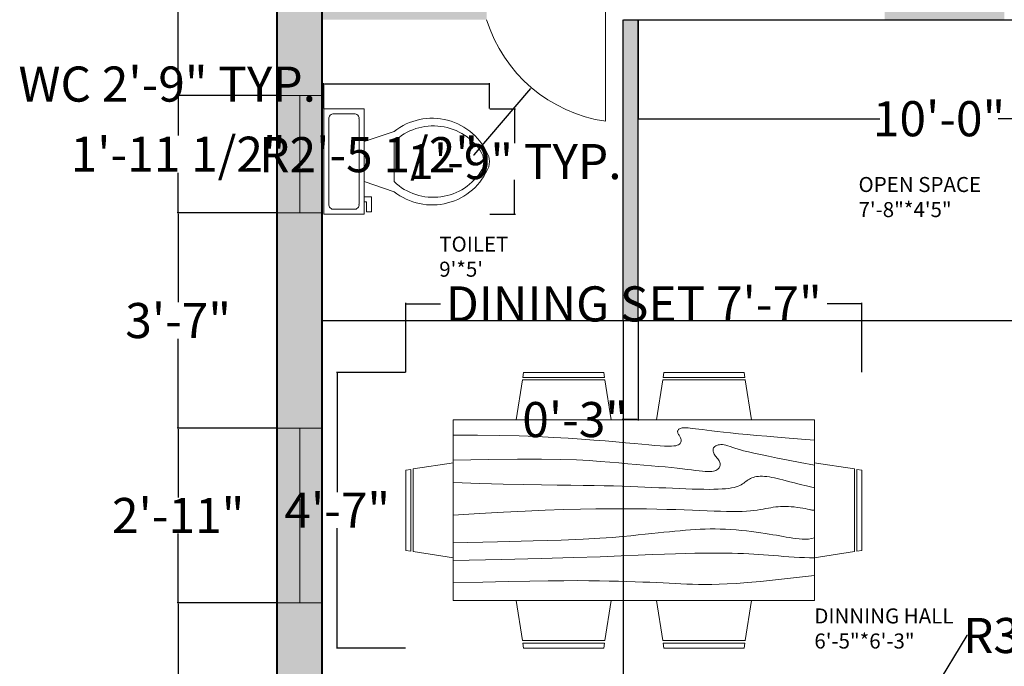
# Model space of a CAD drawing. Units: inches. Extents: x 4466 to 4826, y 3691 to 4152.
# Tile 2 of 4: x 4466 to 4663, y 3859 to 3988. Entities that reach past the tile are written whole.
import ezdxf

# ---------------------------------------------------------------- set-up
doc = ezdxf.new("R2010")
doc.units = ezdxf.units.IN
doc.header["$MEASUREMENT"] = 0
for name, color, linetype, lineweight in [('A-ANNO-DIMS', 2, 'Continuous', 13), ('A-DOOR', 3, 'Continuous', 18), ('A-FLOR-FIXT', 8, 'Continuous', 18), ('A-GLAZ', 4, 'Continuous', 13), ('A-GLAZ-PATT', 9, 'Continuous', 13), ('A-TEXT-ROOM', 7, 'Continuous', 18), ('A-WALL-EXTR', 7, 'Continuous', 40), ('A-WALL-INTR', 7, 'Continuous', 25), ('A-WALL-PATT', 251, 'Continuous', 13)]:
    doc.layers.add(name, color=color, linetype=linetype, lineweight=lineweight)
doc.styles.get("Standard").update_dxf_attribs({"font": 'arial.ttf'})
doc.dimstyles.get("Standard").update_dxf_attribs({"dimtxt": 7, "dimasz": 0.18, "dimexe": 0.18, "dimexo": 0.0625, "dimgap": 0.09, "dimtad": 0, "dimtih": 1, "dimtoh": 1, "dimdec": 0, "dimzin": 0, "dimdsep": 46, "dimlunit": 3, "dimtxsty": 'Standard', "dimcen": 0.09, "dimadec": 0, "dimazin": 0, "dimtfac": 1, "dimtdec": 0, "dimtofl": 0, "dimtmove": 0, "dimatfit": 3, "dimfxl": 1, "dimtolj": 1, "dimtzin": 0, "dimarcsym": 0})

# ---------------------------------------------------------------- blocks, each defined once
blk = doc.blocks.new('Dining Set - 36 x 72 in.')
for p, q in [((-22, 27.5), (-22.1562, 26.50042)), ((-22, 27.5), (-6, 27.5)), ((-5.8437, 26.49966), (-6, 27.5)), ((6, 27.5), (5.8438, 26.50042)), ((6, 27.5), (22, 27.5)), ((22.1563, 26.49966), (22, 27.5)), ((-22.2343, 26.00059), (-23.4847, 17.99762)), ((-22.2304, 26), (-5.7608, 26)), ((-5.8416, 26.5), (-22.1534, 26.5)), ((-4.5152, 17.99762), (-5.7655, 25.99926)), ((5.7657, 26.00059), (4.5153, 17.99762)), ((5.7696, 26), (22.2392, 26)), ((22.1584, 26.5), (5.8466, 26.5)), ((23.4848, 17.99762), (22.2345, 25.99926)), ((36, 18), (-36, 18)), ((-36, 18), (-36, -18)), ((36, -18), (36, 18)), ((-45.5, 8), (-44.5004, 8.15617)), ((-45.5, 8), (-45.5, -8)), ((-44.5, -8.15843), (-44.5, 8.15338)), ((-44.0006, 8.23428), (-35.9976, 9.48474)), ((-44, 8.23041), (-44, -8.23915)), ((44.0006, 8.23428), (35.9976, 9.48474)), ((44, 8.23041), (44, -8.23915)), ((44.5, -8.15843), (44.5, 8.15338)), ((45.5, 8), (44.5005, 8.15617)), ((45.5, 8), (45.5, -8)), ((-44.4997, -8.15631), (-45.5, -8)), ((-35.9976, -9.48476), (-43.9993, -8.2345)), ((35.9976, -9.48476), (43.9993, -8.2345)), ((44.4997, -8.15631), (45.5, -8)), ((-36, -18), (36, -18)), ((-22.2343, -26.0006), (-23.4847, -17.99762)), ((-4.5152, -17.99762), (-5.7655, -25.99928)), ((5.7657, -26.0006), (4.5153, -17.99762)), ((23.4848, -17.99762), (22.2345, -25.99928)), ((-22.2304, -26), (-5.7608, -26)), ((-22, -27.5), (-22.1562, -26.50044)), ((-5.8416, -26.5), (-22.1534, -26.5)), ((-5.8437, -26.49967), (-6, -27.5)), ((5.7696, -26), (22.2392, -26)), ((6, -27.5), (5.8438, -26.50044)), ((22.1584, -26.5), (5.8466, -26.5)), ((22.1563, -26.49967), (22, -27.5)), ((-22, -27.5), (-6, -27.5)), ((6, -27.5), (22, -27.5))]:
    blk.add_line(p, q)
for points in [[(-36, 15), (-31.1772, 14.97754), (-26.8079, 14.91406), (-22.8538, 14.81543), (-19.276, 14.6875), (-16.0362, 14.53613), (-13.0957, 14.36718), (-10.4159, 14.18652), (-7.9583, 14), (-5.6904, 13.81315), (-3.6035, 13.63021), (-1.6954, 13.45508), (0.0365, 13.29166), (1.5945, 13.14388), (2.9811, 13.01562), (4.1988, 12.9108), (5.25, 12.83333), (6.1393, 12.78613), (6.8802, 12.76823), (7.4883, 12.77767), (7.9792, 12.8125), (8.3685, 12.87077), (8.6719, 12.95052), (8.9049, 13.0498), (9.0833, 13.16666), (9.2205, 13.29899), (9.3216, 13.44401), (9.3895, 13.59879), (9.4271, 13.76041), (9.4373, 13.92594), (9.4232, 14.09245), (9.3875, 14.257), (9.3333, 14.41666), (9.2638, 14.56917), (9.1836, 14.71484), (9.0975, 14.85465), (9.0104, 14.98958), (8.9272, 15.1206), (8.8529, 15.2487), (8.7922, 15.37483), (8.75, 15.5), (8.7305, 15.62467), (8.7344, 15.74739), (8.7617, 15.86621), (8.8125, 15.97916), (8.8867, 16.08431), (8.9844, 16.17968), (9.1055, 16.26334), (9.25, 16.33333), (9.4189, 16.38802), (9.6172, 16.42708), (9.8506, 16.45052), (10.125, 16.45833), (10.4463, 16.45052), (10.8203, 16.42708), (11.2529, 16.38802), (11.75, 16.33333), (12.3184, 16.26318), (12.9694, 16.17838), (13.7151, 16.07991), (14.5677, 15.96875), (15.5395, 15.84586), (16.6426, 15.71224), (17.8893, 15.56884), (19.2917, 15.41666), (20.859, 15.25667), (22.5879, 15.08984), (24.4721, 14.91715), (26.5052, 14.73958), (28.6809, 14.5581), (30.9929, 14.3737), (33.4347, 14.18733), (36, 14)], [(-36, 10), (-28.9766, 10.14274), (-23.1725, 10.20442), (-18.4241, 10.19775), (-14.5677, 10.13541), (-11.4399, 10.03011), (-8.877, 9.89453), (-6.7154, 9.74137), (-4.7917, 9.58333), (-2.9698, 9.43082), (-1.2246, 9.28515), (0.4415, 9.14534), (2.026, 9.01041), (3.5266, 8.87939), (4.9408, 8.7513), (6.266, 8.62516), (7.5, 8.5), (8.6411, 8.37549), (9.6914, 8.2539), (10.6538, 8.13818), (11.5312, 8.03125), (12.3267, 7.93603), (13.043, 7.85547), (13.6831, 7.79248), (14.25, 7.75), (14.7471, 7.7303), (15.1797, 7.73307), (15.5537, 7.75732), (15.875, 7.80208), (16.1494, 7.86637), (16.3828, 7.94922), (16.5811, 8.04964), (16.75, 8.16666), (16.8944, 8.29915), (17.0143, 8.44531), (17.1089, 8.60319), (17.1771, 8.77083), (17.218, 8.94629), (17.2305, 9.1276), (17.2137, 9.31282), (17.1667, 9.5), (17.0895, 9.6875), (16.987, 9.875), (16.8649, 10.0625), (16.7292, 10.25), (16.5856, 10.4375), (16.4401, 10.625), (16.2985, 10.8125), (16.1667, 11), (16.05, 11.18733), (15.9518, 11.3737), (15.8752, 11.5581), (15.8229, 11.73958), (15.798, 11.91715), (15.8034, 12.08984), (15.842, 12.25667), (15.9167, 12.41666), (16.0295, 12.56836), (16.1784, 12.70833), (16.3605, 12.83268), (16.5729, 12.9375), (16.8127, 13.01888), (17.0768, 13.07291), (17.3625, 13.0957), (17.6667, 13.08333), (17.9894, 13.03312), (18.3418, 12.94726), (18.7382, 12.82918), (19.1927, 12.68229), (19.7195, 12.51001), (20.3327, 12.31575), (21.0465, 12.10294), (21.875, 11.875), (22.8357, 11.63354), (23.959, 11.37304), (25.2786, 11.08618), (26.8282, 10.76562), (28.6414, 10.40405), (30.752, 9.99414), (33.1936, 9.52856), (36, 9)], [(-36, 5.5), (-30.7157, 5.3348), (-26.069, 5.20963), (-21.9946, 5.11767), (-18.4271, 5.05208), (-15.3009, 5.00602), (-12.5508, 4.97265), (-10.1112, 4.94515), (-7.9167, 4.91666), (-5.909, 4.88167), (-4.0586, 4.83984), (-2.3429, 4.79215), (-0.7396, 4.73958), (0.7739, 4.6831), (2.22, 4.6237), (3.6213, 4.56233), (5, 4.5), (6.373, 4.43782), (7.7344, 4.3776), (9.0723, 4.32129), (10.375, 4.27083), (11.6309, 4.22819), (12.8281, 4.19531), (13.9551, 4.17415), (15, 4.16666), (15.954, 4.17448), (16.819, 4.19791), (17.6001, 4.23698), (18.3021, 4.29166), (18.9299, 4.36198), (19.4883, 4.44791), (19.9823, 4.54948), (20.4167, 4.66666), (20.7969, 4.79899), (21.1302, 4.94401), (21.4245, 5.09879), (21.6875, 5.26041), (21.9271, 5.42594), (22.1511, 5.59245), (22.3672, 5.757), (22.5834, 5.91666), (22.8065, 6.06868), (23.0404, 6.21093), (23.2879, 6.34147), (23.5521, 6.45833), (23.8358, 6.55957), (24.142, 6.64323), (24.4735, 6.70735), (24.8334, 6.75), (25.2235, 6.76969), (25.642, 6.76692), (26.0858, 6.74267), (26.5521, 6.69791), (27.0379, 6.63362), (27.5404, 6.55078), (28.0565, 6.45036), (28.5834, 6.33333), (29.1242, 6.19987), (29.7071, 6.04687), (30.3661, 5.87044), (31.1354, 5.66666), (32.0493, 5.43164), (33.142, 5.16146), (34.4475, 4.85221), (36, 4.5)], [(-36, -1), (-30.7915, -0.6591), (-26.0195, -0.38216), (-21.6519, -0.16284), (-17.6563, 0.00521), (-14.0005, 0.12833), (-10.6523, 0.21289), (-7.5796, 0.26522), (-4.75, 0.29166), (-2.134, 0.29793), (0.2878, 0.28711), (2.5317, 0.26163), (4.6146, 0.22396), (6.5529, 0.17651), (8.3633, 0.12174), (10.0623, 0.06209), (11.6667, 0), (13.1899, -0.06201), (14.6341, -0.1211), (15.9982, -0.17432), (17.2813, -0.21875), (18.4823, -0.25147), (19.6003, -0.26953), (20.6343, -0.27002), (21.5834, -0.25), (22.4481, -0.20768), (23.2357, -0.14584), (23.9549, -0.06836), (24.6146, 0.02083), (25.2235, 0.11784), (25.7904, 0.21875), (26.3241, 0.31966), (26.8334, 0.41666), (27.3265, 0.50618), (27.8099, 0.58593), (28.2894, 0.65397), (28.7709, 0.70833), (29.2601, 0.74707), (29.763, 0.76823), (30.2855, 0.76985), (30.8334, 0.75), (31.4088, 0.70784), (31.9994, 0.64713), (32.589, 0.57275), (33.1615, 0.48958), (33.7008, 0.4025), (34.1908, 0.3164), (34.6153, 0.23616), (34.9584, 0.16666), (35.2099, 0.11165), (35.3848, 0.07031), (35.504, 0.04069), (35.5886, 0.02083), (35.6594, 0.00879), (35.7377, 0.0026), (35.8442, 0.00032), (36, 0)], [(-36, -6.5), (-27.1843, -6.31267), (-20.084, -6.1263), (-14.469, -5.9419), (-10.1094, -5.76042), (-6.7752, -5.58285), (-4.2363, -5.41016), (-2.2629, -5.24333), (-0.625, -5.08334), (0.8708, -4.93099), (2.2715, -4.78646), (3.5872, -4.64974), (4.8281, -4.52084), (6.0046, -4.39974), (7.127, -4.28646), (8.2053, -4.18099), (9.25, -4.08334), (10.2705, -3.99382), (11.2734, -3.91407), (12.2647, -3.84603), (13.25, -3.79167), (14.2354, -3.75293), (15.2266, -3.73177), (16.2295, -3.73015), (17.25, -3.75), (18.2912, -3.79248), (19.3451, -3.85547), (20.4009, -3.93604), (21.4479, -4.03125), (22.4754, -4.13819), (23.4727, -4.25391), (24.4289, -4.37549), (25.3334, -4.5), (26.1785, -4.62492), (26.9694, -4.74935), (27.7145, -4.87281), (28.4219, -4.99479), (29.1, -5.11483), (29.7572, -5.23242), (30.4016, -5.34709), (31.0417, -5.45834), (31.6837, -5.56437), (32.3262, -5.65821), (32.9658, -5.73153), (33.599, -5.77604), (34.2224, -5.78345), (34.8327, -5.74545), (35.4264, -5.65373), (36, -5.5)], [(-36, -10), (-26.4022, -9.81299), (-18.4675, -9.62891), (-11.9839, -9.45069), (-6.7396, -9.28125), (-2.5226, -9.12354), (0.8789, -8.98047), (3.6769, -8.85498), (6.0833, -8.75), (8.2767, -8.66765), (10.3021, -8.60677), (12.1712, -8.56543), (13.8958, -8.54167), (15.4876, -8.53353), (16.9583, -8.53907), (18.3197, -8.55632), (19.5834, -8.58334), (20.7616, -8.61841), (21.8685, -8.66081), (22.9188, -8.71004), (23.9271, -8.76563), (24.9081, -8.82707), (25.8763, -8.89388), (26.8465, -8.96558), (27.8334, -9.04167), (28.8474, -9.12118), (29.8828, -9.20117), (30.93, -9.27824), (31.9792, -9.34896), (33.0205, -9.40991), (34.0443, -9.45768), (35.0407, -9.48885), (36, -9.5)], [(-36, -14.5), (-30.0881, -14.33513), (-25.0332, -14.21224), (-20.7312, -14.12647), (-17.0781, -14.07292), (-13.97, -14.04671), (-11.3027, -14.04297), (-8.9724, -14.05681), (-6.875, -14.08334), (-4.9224, -14.11833), (-3.0905, -14.16016), (-1.3709, -14.20785), (0.2448, -14.26042), (1.7647, -14.3169), (3.1973, -14.3763), (4.5507, -14.43767), (5.8333, -14.5), (7.0554, -14.5621), (8.235, -14.62175), (9.3922, -14.67652), (10.5469, -14.72396), (11.7192, -14.76164), (12.929, -14.78711), (14.1965, -14.79794), (15.5417, -14.79167), (16.9933, -14.76424), (18.6152, -14.70508), (20.4804, -14.60197), (22.6615, -14.44271), (25.2312, -14.21509), (28.2624, -13.9069), (31.8277, -13.50594), (36, -13)]]:
    blk.add_lwpolyline(points)
blk = doc.blocks.new('Toilet - top')
for p, q in [((9.5, -6), (9.5, -2)), ((-10, -8.5), (-8, -8.5)), ((-10, -9.5), (-10, -8.5)), ((-7, -9.5), (-10, -9.5)), ((-8, -8.5), (-8, -8)), ((-7, -8), (-7, -9.5)), ((-4, -8), (-6, -14)), ((4, -8), (6, -14)), ((4, -14), (-4, -14))]:
    blk.add_line(p, q)
blk.add_lwpolyline([(10.5, -8), (10.5, 0), (-10.5, 0), (-10.5, -8)], close=True)
for points in [[(8.5, -1), (-8.5, -1)], [(-9.5, -2), (-9.5, -6)], [(-8.5, -7), (8.5, -7)]]:
    blk.add_lwpolyline(points)
for centre, radius, start, end in [((-8.62, -1.88), 0.884, 81.8699, 188.1301), ((8.62, -1.88), 0.884, 351.8699, 98.1301), ((-8.62, -6.12), 0.884, 171.8699, 278.1301), ((8.62, -6.12), 0.884, 261.8699, 8.1301), ((3.52, -21.58), 12.17, 141.4691, 247.9714), ((4.2, -21.82), 11.33, 136.3677, 238.9468), ((-3.52, -21.58), 12.17, 292.0284, 38.5307), ((-4.2, -21.82), 11.33, 301.053, 43.6321), ((0, -27.88), 4, 245.7318, 294.2682), ((0, -29), 4, 254.8605, 285.1395)]:
    blk.add_arc(centre, radius, start, end)
blk = doc.blocks.new('*D10')
at = {"layer": 'A-ANNO-DIMS', "color": 0, "lineweight": -2, "transparency": 16777216}
for p, q in [((4527.05, 3975.44), (4526.87, 3975.44)), ((4527.05, 3970.54), (4527.05, 3975.62)), ((4559.92, 3975.44), (4527.23, 3975.44)), ((4560.1, 3970.54), (4560.1, 3975.62))]:
    blk.add_line(p, q, dxfattribs=at)
at = {"layer": 'A-ANNO-DIMS', "color": 0, "transparency": 16777216}
for points in [[(4527.23, 3975.47), (4527.23, 3975.41), (4527.05, 3975.44)], [(4559.92, 3975.47), (4559.92, 3975.41), (4560.1, 3975.44)]]:
    blk.add_solid(points, dxfattribs=at)
at = {"layer": 'Defpoints', "color": 0, "transparency": 16777216}
for p in [(4527.05, 3975.44), (4527.05, 3970.48), (4560.1, 3970.48)]:
    blk.add_point(p, dxfattribs=at)
at = {"layer": 'A-ANNO-DIMS', "color": 0, "transparency": 16777216, "insert": (4495.8, 3975.44), "char_height": 7, "attachment_point": 5}
blk.add_mtext('\\A1;WC 2\'-9" TYP.', dxfattribs=at)
blk = doc.blocks.new('*D11')
at = {"layer": 'A-ANNO-DIMS', "color": 0, "lineweight": -2, "transparency": 16777216}
for p, q in [((4560.16, 3970.48), (4565.23, 3970.48)), ((4565.05, 3970.3), (4565.05, 3963.64)), ((4565.05, 3949.66), (4565.05, 3956.32)), ((4560.16, 3949.48), (4565.23, 3949.48))]:
    blk.add_line(p, q, dxfattribs=at)
at = {"layer": 'A-ANNO-DIMS', "color": 0, "transparency": 16777216}
for points in [[(4565.02, 3970.3), (4565.08, 3970.3), (4565.05, 3970.48)], [(4565.02, 3949.66), (4565.08, 3949.66), (4565.05, 3949.48)]]:
    blk.add_solid(points, dxfattribs=at)
at = {"layer": 'Defpoints', "color": 0, "transparency": 16777216}
for p in [(4560.1, 3970.48), (4565.05, 3970.48), (4560.1, 3949.48)]:
    blk.add_point(p, dxfattribs=at)
at = {"layer": 'A-ANNO-DIMS', "color": 0, "transparency": 16777216, "insert": (4565.05, 3959.98), "char_height": 7, "attachment_point": 5}
blk.add_mtext('\\A1;1\'-9" TYP.', dxfattribs=at)
blk = doc.blocks.new('*D12')
at = {"layer": 'A-ANNO-DIMS', "color": 0, "lineweight": -2, "transparency": 16777216}
for p, q in [((4543.36, 3918.01), (4543.36, 3931.78)), ((4543.54, 3931.6), (4550.3, 3931.6)), ((4634.18, 3931.6), (4627.41, 3931.6)), ((4634.36, 3918.01), (4634.36, 3931.78))]:
    blk.add_line(p, q, dxfattribs=at)
at = {"layer": 'A-ANNO-DIMS', "color": 0, "transparency": 16777216}
for points in [[(4543.54, 3931.63), (4543.54, 3931.57), (4543.36, 3931.6)], [(4634.18, 3931.63), (4634.18, 3931.57), (4634.36, 3931.6)]]:
    blk.add_solid(points, dxfattribs=at)
at = {"layer": 'Defpoints', "color": 0, "transparency": 16777216}
for p in [(4634.36, 3931.6), (4543.36, 3917.95), (4634.36, 3917.95)]:
    blk.add_point(p, dxfattribs=at)
at = {"layer": 'A-ANNO-DIMS', "color": 0, "transparency": 16777216, "insert": (4588.86, 3931.6), "char_height": 7, "attachment_point": 5}
blk.add_mtext('\\A1;DINING SET 7\'-7"', dxfattribs=at)
blk = doc.blocks.new('*D13')
at = {"layer": 'A-ANNO-DIMS', "color": 0, "lineweight": -2, "transparency": 16777216}
for p, q in [((4543.29, 3917.95), (4529.53, 3917.95)), ((4529.71, 3917.77), (4529.71, 3894.04)), ((4529.71, 3863.13), (4529.71, 3886.86)), ((4543.29, 3862.95), (4529.53, 3862.95))]:
    blk.add_line(p, q, dxfattribs=at)
at = {"layer": 'A-ANNO-DIMS', "color": 0, "transparency": 16777216}
for points in [[(4529.68, 3917.77), (4529.74, 3917.77), (4529.71, 3917.95)], [(4529.68, 3863.13), (4529.74, 3863.13), (4529.71, 3862.95)]]:
    blk.add_solid(points, dxfattribs=at)
at = {"layer": 'Defpoints', "color": 0, "transparency": 16777216}
for p in [(4529.71, 3917.95), (4543.36, 3917.95), (4543.36, 3862.95)]:
    blk.add_point(p, dxfattribs=at)
at = {"layer": 'A-ANNO-DIMS', "color": 0, "transparency": 16777216, "insert": (4529.71, 3890.45), "char_height": 7, "attachment_point": 5}
blk.add_mtext('\\A1;4\'-7"', dxfattribs=at)
blk = doc.blocks.new('*D22')
at = {"layer": 'A-ANNO-DIMS', "color": 0, "lineweight": -2, "transparency": 16777216}
for p, q in [((4517.67, 3871.98), (4497.8, 3871.98)), ((4497.98, 3871.8), (4497.98, 3854.33)), ((4497.98, 3829.43), (4497.98, 3846.9)), ((4517.67, 3829.25), (4497.8, 3829.25))]:
    blk.add_line(p, q, dxfattribs=at)
at = {"layer": 'A-ANNO-DIMS', "color": 0, "transparency": 16777216}
for points in [[(4497.95, 3871.8), (4498.01, 3871.8), (4497.98, 3871.98)], [(4497.95, 3829.43), (4498.01, 3829.43), (4497.98, 3829.25)]]:
    blk.add_solid(points, dxfattribs=at)
at = {"layer": 'Defpoints', "color": 0, "transparency": 16777216}
for p in [(4497.98, 3871.98), (4517.73, 3871.98), (4517.73, 3829.25)]:
    blk.add_point(p, dxfattribs=at)
at = {"layer": 'A-ANNO-DIMS', "color": 0, "transparency": 16777216, "insert": (4497.98, 3850.62), "char_height": 7, "attachment_point": 5}
blk.add_mtext('\\A1;3\'-6 1/2"', dxfattribs=at)
blk = doc.blocks.new('*D23')
at = {"layer": 'A-ANNO-DIMS', "color": 0, "lineweight": -2, "transparency": 16777216}
for p, q in [((4517.67, 3906.82), (4497.8, 3906.82)), ((4497.98, 3906.64), (4497.98, 3893)), ((4497.98, 3872.16), (4497.98, 3885.79)), ((4517.67, 3871.98), (4497.8, 3871.98))]:
    blk.add_line(p, q, dxfattribs=at)
at = {"layer": 'A-ANNO-DIMS', "color": 0, "transparency": 16777216}
for points in [[(4497.95, 3906.64), (4498.01, 3906.64), (4497.98, 3906.82)], [(4497.95, 3872.16), (4498.01, 3872.16), (4497.98, 3871.98)]]:
    blk.add_solid(points, dxfattribs=at)
at = {"layer": 'Defpoints', "color": 0, "transparency": 16777216}
for p in [(4497.98, 3906.82), (4517.73, 3906.82), (4517.73, 3871.98)]:
    blk.add_point(p, dxfattribs=at)
at = {"layer": 'A-ANNO-DIMS', "color": 0, "transparency": 16777216, "insert": (4497.98, 3889.4), "char_height": 7, "attachment_point": 5}
blk.add_mtext('\\A1;2\'-11"', dxfattribs=at)
blk = doc.blocks.new('*D24')
at = {"layer": 'A-ANNO-DIMS', "color": 0, "lineweight": -2, "transparency": 16777216}
for p, q in [((4517.67, 3949.75), (4497.8, 3949.75)), ((4497.98, 3949.57), (4497.98, 3931.95)), ((4497.98, 3907), (4497.98, 3924.62)), ((4517.67, 3906.82), (4497.8, 3906.82))]:
    blk.add_line(p, q, dxfattribs=at)
at = {"layer": 'A-ANNO-DIMS', "color": 0, "transparency": 16777216}
for points in [[(4497.95, 3949.57), (4498.01, 3949.57), (4497.98, 3949.75)], [(4497.95, 3907), (4498.01, 3907), (4497.98, 3906.82)]]:
    blk.add_solid(points, dxfattribs=at)
at = {"layer": 'Defpoints', "color": 0, "transparency": 16777216}
for p in [(4497.98, 3949.75), (4517.73, 3949.75), (4517.73, 3906.82)]:
    blk.add_point(p, dxfattribs=at)
at = {"layer": 'A-ANNO-DIMS', "color": 0, "transparency": 16777216, "insert": (4497.98, 3928.28), "char_height": 7, "attachment_point": 5}
blk.add_mtext('\\A1;3\'-7"', dxfattribs=at)
blk = doc.blocks.new('*D25')
at = {"layer": 'A-ANNO-DIMS', "color": 0, "lineweight": -2, "transparency": 16777216}
for p, q in [((4517.67, 3973.15), (4497.8, 3973.15)), ((4497.98, 3972.97), (4497.98, 3965.16)), ((4497.98, 3949.93), (4497.98, 3957.74)), ((4517.67, 3949.75), (4497.8, 3949.75))]:
    blk.add_line(p, q, dxfattribs=at)
at = {"layer": 'A-ANNO-DIMS', "color": 0, "transparency": 16777216}
for points in [[(4497.95, 3972.97), (4498.01, 3972.97), (4497.98, 3973.15)], [(4497.95, 3949.93), (4498.01, 3949.93), (4497.98, 3949.75)]]:
    blk.add_solid(points, dxfattribs=at)
at = {"layer": 'Defpoints', "color": 0, "transparency": 16777216}
for p in [(4497.98, 3973.15), (4517.73, 3973.15), (4517.73, 3949.75)]:
    blk.add_point(p, dxfattribs=at)
at = {"layer": 'A-ANNO-DIMS', "color": 0, "transparency": 16777216, "insert": (4497.98, 3961.45), "char_height": 7, "attachment_point": 5}
blk.add_mtext('\\A1;1\'-11 1/2"', dxfattribs=at)
blk = doc.blocks.new('*D26')
at = {"layer": 'A-ANNO-DIMS', "color": 0, "lineweight": -2, "transparency": 16777216}
for p, q in [((4517.67, 4027.88), (4497.8, 4027.88)), ((4497.98, 4027.7), (4497.98, 4004.23)), ((4497.98, 3973.33), (4497.98, 3996.81)), ((4517.67, 3973.15), (4497.8, 3973.15))]:
    blk.add_line(p, q, dxfattribs=at)
at = {"layer": 'A-ANNO-DIMS', "color": 0, "transparency": 16777216}
for points in [[(4497.95, 4027.7), (4498.01, 4027.7), (4497.98, 4027.88)], [(4497.95, 3973.33), (4498.01, 3973.33), (4497.98, 3973.15)]]:
    blk.add_solid(points, dxfattribs=at)
at = {"layer": 'Defpoints', "color": 0, "transparency": 16777216}
for p in [(4497.98, 4027.88), (4517.73, 4027.88), (4517.73, 3973.15)]:
    blk.add_point(p, dxfattribs=at)
at = {"layer": 'A-ANNO-DIMS', "color": 0, "transparency": 16777216, "insert": (4497.98, 4000.52), "char_height": 7, "attachment_point": 5}
blk.add_mtext('\\A1;4\'-6 1/2"', dxfattribs=at)
blk = doc.blocks.new('*D41')
at = {"layer": 'A-ANNO-DIMS', "color": 0, "lineweight": -2, "transparency": 16777216}
for p, q in [((4526.73, 3928.22), (4526.73, 3740.35)), ((4586.73, 3928.22), (4586.73, 3740.35)), ((4526.91, 3740.53), (4547.34, 3740.53)), ((4586.55, 3740.53), (4566.13, 3740.53))]:
    blk.add_line(p, q, dxfattribs=at)
at = {"layer": 'A-ANNO-DIMS', "color": 0, "transparency": 16777216}
for points in [[(4526.91, 3740.56), (4526.91, 3740.5), (4526.73, 3740.53)], [(4586.55, 3740.56), (4586.55, 3740.5), (4586.73, 3740.53)]]:
    blk.add_solid(points, dxfattribs=at)
at = {"layer": 'Defpoints', "color": 0, "transparency": 16777216}
for p in [(4526.73, 3928.28), (4586.73, 3928.28), (4586.73, 3740.53)]:
    blk.add_point(p, dxfattribs=at)
at = {"layer": 'A-ANNO-DIMS', "color": 0, "transparency": 16777216, "insert": (4556.73, 3740.53), "char_height": 7, "attachment_point": 5}
blk.add_mtext('\\A1;5\'-0"', dxfattribs=at)
blk = doc.blocks.new('*D42')
at = {"layer": 'A-ANNO-DIMS', "color": 0, "lineweight": -2, "transparency": 16777216}
for p, q in [((4586.8, 3988.28), (4801.66, 3988.28)), ((4801.48, 3988.1), (4801.48, 3961.94)), ((4801.48, 3928.46), (4801.48, 3954.62)), ((4586.8, 3928.28), (4801.66, 3928.28))]:
    blk.add_line(p, q, dxfattribs=at)
at = {"layer": 'A-ANNO-DIMS', "color": 0, "transparency": 16777216}
for points in [[(4801.45, 3988.1), (4801.51, 3988.1), (4801.48, 3988.28)], [(4801.45, 3928.46), (4801.51, 3928.46), (4801.48, 3928.28)]]:
    blk.add_solid(points, dxfattribs=at)
at = {"layer": 'Defpoints', "color": 0, "transparency": 16777216}
for p in [(4586.73, 3988.28), (4801.48, 3988.28), (4586.73, 3928.28)]:
    blk.add_point(p, dxfattribs=at)
at = {"layer": 'A-ANNO-DIMS', "color": 0, "transparency": 16777216, "insert": (4801.48, 3958.28), "char_height": 7, "attachment_point": 5}
blk.add_mtext('\\A1;5\'-0"', dxfattribs=at)
blk = doc.blocks.new('*D43')
at = {"layer": 'A-ANNO-DIMS', "color": 0, "lineweight": -2, "transparency": 16777216}
for p, q in [((4586.73, 3928.22), (4586.73, 3908.35)), ((4589.73, 3928.22), (4589.73, 3908.35)), ((4586.73, 3908.53), (4586.55, 3908.53)), ((4589.55, 3908.53), (4586.91, 3908.53))]:
    blk.add_line(p, q, dxfattribs=at)
at = {"layer": 'A-ANNO-DIMS', "color": 0, "transparency": 16777216}
for points in [[(4586.91, 3908.56), (4586.91, 3908.5), (4586.73, 3908.53)], [(4589.55, 3908.56), (4589.55, 3908.5), (4589.73, 3908.53)]]:
    blk.add_solid(points, dxfattribs=at)
at = {"layer": 'Defpoints', "color": 0, "transparency": 16777216}
for p in [(4586.73, 3928.28), (4589.73, 3928.28), (4586.73, 3908.53)]:
    blk.add_point(p, dxfattribs=at)
at = {"layer": 'A-ANNO-DIMS', "color": 0, "transparency": 16777216, "insert": (4577.16, 3908.53), "char_height": 7, "attachment_point": 5}
blk.add_mtext('\\A1;0\'-3"', dxfattribs=at)
blk = doc.blocks.new('*D55')
at = {"layer": 'A-ANNO-DIMS', "color": 0, "lineweight": -2, "transparency": 16777216}
for p, q in [((4589.73, 3988.22), (4589.73, 3968.35)), ((4709.73, 3988.22), (4709.73, 3968.35)), ((4589.91, 3968.53), (4637.95, 3968.53)), ((4709.55, 3968.53), (4661.52, 3968.53))]:
    blk.add_line(p, q, dxfattribs=at)
at = {"layer": 'A-ANNO-DIMS', "color": 0, "transparency": 16777216}
for points in [[(4589.91, 3968.56), (4589.91, 3968.5), (4589.73, 3968.53)], [(4709.55, 3968.56), (4709.55, 3968.5), (4709.73, 3968.53)]]:
    blk.add_solid(points, dxfattribs=at)
at = {"layer": 'Defpoints', "color": 0, "transparency": 16777216}
for p in [(4589.73, 3988.28), (4709.73, 3988.28), (4589.73, 3968.53)]:
    blk.add_point(p, dxfattribs=at)
at = {"layer": 'A-ANNO-DIMS', "color": 0, "transparency": 16777216, "insert": (4649.73, 3968.53), "char_height": 7, "attachment_point": 5}
blk.add_mtext('\\A1;10\'-0"', dxfattribs=at)
blk = doc.blocks.new('*D58')
at = {"layer": 'A-ANNO-DIMS', "color": 0, "lineweight": -2, "transparency": 16777216}
for p, q in [((4655.25, 3865.47), (4642.54, 3844.4)), ((4655.43, 3865.47), (4655.25, 3865.47)), ((4621.03, 3808.87), (4621.21, 3808.87)), ((4621.12, 3808.78), (4621.12, 3808.96))]:
    blk.add_line(p, q, dxfattribs=at)
at = {"layer": 'A-ANNO-DIMS', "color": 0, "transparency": 16777216}
blk.add_solid([(4642.52, 3844.41), (4642.57, 3844.38), (4642.45, 3844.24)], dxfattribs=at)
at = {"layer": 'Defpoints', "color": 0, "transparency": 16777216}
for p in [(4642.45, 3844.24), (4621.12, 3808.87)]:
    blk.add_point(p, dxfattribs=at)
at = {"layer": 'A-ANNO-DIMS', "color": 0, "transparency": 16777216, "insert": (4676.33, 3865.47), "char_height": 7, "attachment_point": 5}
blk.add_mtext('\\A1;R3\'-5 1/2"', dxfattribs=at)
blk = doc.blocks.new('*D63')
at = {"layer": 'A-ANNO-DIMS', "color": 0, "lineweight": -2, "transparency": 16777216}
for p, q in [((4587.35, 3996.99), (4587.53, 3996.99)), ((4587.44, 3996.9), (4587.44, 3997.08)), ((4557.04, 3961.36), (4568.32, 3974.59)), ((4556.86, 3961.36), (4557.04, 3961.36))]:
    blk.add_line(p, q, dxfattribs=at)
at = {"layer": 'A-ANNO-DIMS', "color": 0, "transparency": 16777216}
blk.add_solid([(4568.3, 3974.6), (4568.35, 3974.57), (4568.44, 3974.72)], dxfattribs=at)
at = {"layer": 'Defpoints', "color": 0, "transparency": 16777216}
for p in [(4587.44, 3996.99), (4568.44, 3974.72)]:
    blk.add_point(p, dxfattribs=at)
at = {"layer": 'A-ANNO-DIMS', "color": 0, "transparency": 16777216, "insert": (4535.96, 3961.36), "char_height": 7, "attachment_point": 5}
blk.add_mtext('\\A1;R2\'-5 1/2"', dxfattribs=at)

msp = doc.modelspace()

# ---------------------------------------------------------------- hatches: boundary and pattern name
at = {"layer": 'A-GLAZ-PATT'}
h = msp.add_hatch(color=256, dxfattribs=at)
h.dxf.hatch_style = 1
h.paths.add_polyline_path([(4781.73, 3815.6), (4777.23, 3815.6), (4777.23, 3780.77), (4781.73, 3780.77)])
h.paths.add_polyline_path([(4777.23, 3815.6), (4772.73, 3815.6), (4772.73, 3780.77), (4777.23, 3780.77)])
h.paths.add_polyline_path([(4781.73, 3906.43), (4777.23, 3906.43), (4777.23, 3867), (4781.73, 3867)])
h.paths.add_polyline_path([(4777.23, 3906.43), (4772.73, 3906.43), (4772.73, 3867), (4777.23, 3867)])
h.paths.add_polyline_path([(4777.23, 3975.56), (4772.73, 3975.56), (4772.73, 3940.28), (4777.23, 3940.28)])
h.paths.add_polyline_path([(4781.73, 3975.56), (4777.23, 3975.56), (4777.23, 3940.28), (4781.73, 3940.28)])
h.paths.add_polyline_path([(4781.73, 4086.44), (4777.23, 4086.44), (4777.23, 4025.83), (4781.73, 4025.83)])
h.paths.add_polyline_path([(4777.23, 4086.44), (4772.73, 4086.44), (4772.73, 4025.83), (4777.23, 4025.83)])
h.paths.add_polyline_path([(4526.73, 4085.19), (4522.23, 4085.19), (4522.23, 4027.88), (4526.73, 4027.88)])
h.paths.add_polyline_path([(4522.23, 4085.19), (4517.73, 4085.19), (4517.73, 4027.88), (4522.23, 4027.88)])
h.paths.add_polyline_path([(4526.73, 3973.15), (4522.23, 3973.15), (4522.23, 3949.75), (4526.73, 3949.75)])
h.paths.add_polyline_path([(4522.23, 3973.15), (4517.73, 3973.15), (4517.73, 3949.75), (4522.23, 3949.75)])
h.paths.add_polyline_path([(4522.23, 3906.82), (4517.73, 3906.82), (4517.73, 3871.98), (4522.23, 3871.98)])
h.paths.add_polyline_path([(4526.73, 3906.82), (4522.23, 3906.82), (4522.23, 3871.98), (4526.73, 3871.98)])
h.paths.add_polyline_path([(4526.73, 3829.25), (4522.23, 3829.25), (4522.23, 3789.34), (4526.73, 3789.34)])
h.paths.add_polyline_path([(4522.23, 3829.25), (4517.73, 3829.25), (4517.73, 3789.34), (4522.23, 3789.34)])
at = {"layer": 'A-WALL-PATT'}
h = msp.add_hatch(color=256, dxfattribs=at)
h.dxf.hatch_style = 1
h.paths.add_polyline_path([(4781.73, 4120.28), (4517.73, 4120.28), (4517.73, 4085.19), (4526.73, 4085.19), (4526.73, 4111.28), (4772.73, 4111.28), (4772.73, 4086.44), (4781.73, 4086.44)])
h.paths.add_polyline_path([(4526.73, 4027.88), (4517.73, 4027.88), (4517.73, 3973.15), (4526.73, 3973.15)])
h.paths.add_polyline_path([(4781.73, 4025.83), (4772.73, 4025.83), (4772.73, 3975.56), (4781.73, 3975.56)])
h.paths.add_polyline_path([(4651.73, 4111.28), (4647.73, 4111.28), (4647.73, 3991.28), (4638.9, 3991.28), (4638.9, 3988.28), (4662.75, 3988.28), (4662.75, 3991.28), (4651.73, 3991.28)])
h.paths.add_polyline_path([(4781.73, 3780.77), (4772.73, 3780.77), (4772.73, 3769.28), (4657.39, 3769.28), (4657.39, 3760.28), (4781.73, 3760.28)])
h.paths.add_polyline_path([(4781.73, 3867), (4772.73, 3867), (4772.73, 3815.6), (4781.73, 3815.6)])
h.paths.add_polyline_path([(4781.73, 3940.28), (4772.73, 3940.28), (4772.73, 3906.43), (4781.73, 3906.43)])
h.paths.add_polyline_path([(4526.73, 3949.75), (4517.73, 3949.75), (4517.73, 3906.82), (4526.73, 3906.82)])
h.paths.add_polyline_path([(4526.73, 3871.98), (4517.73, 3871.98), (4517.73, 3829.25), (4526.73, 3829.25)])
h.paths.add_polyline_path([(4618.18, 3769.28), (4526.73, 3769.28), (4526.73, 3789.34), (4517.73, 3789.34), (4517.73, 3760.28), (4618.18, 3760.28)])
h.paths.add_polyline_path([(4576.17, 3850.28), (4526.73, 3850.28), (4526.73, 3847.28), (4576.17, 3847.28)])
h.paths.add_polyline_path([(4613.73, 3825.64), (4618.18, 3825.64), (4618.18, 3828.64), (4613.73, 3828.64), (4613.73, 3850.28), (4610.73, 3850.28), (4606.34, 3850.28), (4606.34, 3847.28), (4610.73, 3847.28), (4610.73, 3769.28), (4613.73, 3769.28)])
h.paths.add_polyline_path([(4772.73, 3828.64), (4657.39, 3828.64), (4657.39, 3825.64), (4772.73, 3825.64)])
h.paths.add_polyline_path([(4589.73, 3988.28), (4586.73, 3988.28), (4586.73, 3928.28), (4589.73, 3928.28)])
h.paths.add_polyline_path([(4712.73, 3956.78), (4709.73, 3956.78), (4709.73, 3925.28), (4772.73, 3925.28), (4772.73, 3928.28), (4712.73, 3928.28)])
h.paths.add_polyline_path([(4772.73, 3991.28), (4705.82, 3991.28), (4705.82, 3988.28), (4772.73, 3988.28)])
h.paths.add_polyline_path([(4559.49, 3991.28), (4526.73, 3991.28), (4526.73, 3988.28), (4559.49, 3988.28)])

# ---------------------------------------------------------------- linework, layer by layer
at = {"layer": 'A-DOOR'}
for q in [(4583.24, 3991.28), (4583.24, 3968.02)]:
    msp.add_line((4583.24, 3988.28), q, dxfattribs=at)
msp.add_arc((4587.44, 3996.99), 29.27, 197.3221, 261.7576, dxfattribs=at)
at = {"layer": 'A-GLAZ'}
for p, q in [((4517.73, 3973.15), (4526.73, 3973.15)), ((4522.23, 3973.15), (4522.23, 3949.75)), ((4517.73, 3949.75), (4526.73, 3949.75)), ((4517.73, 3906.82), (4526.73, 3906.82)), ((4522.23, 3906.82), (4522.23, 3871.98)), ((4517.73, 3871.98), (4526.73, 3871.98))]:
    msp.add_line(p, q, dxfattribs=at)
at = {"layer": 'A-WALL-EXTR'}
msp.add_line((4526.73, 3769.28), (4526.73, 4111.28), dxfattribs=at)
msp.add_lwpolyline([(4618.18, 3760.28), (4517.73, 3760.28), (4517.73, 4120.28), (4781.73, 4120.28), (4781.73, 3760.28), (4657.39, 3760.28)], dxfattribs=at)
at = {"layer": 'A-WALL-INTR'}
for p, q in [((4586.73, 3928.28), (4586.73, 3988.28)), ((4589.73, 3928.28), (4589.73, 3988.28)), ((4638.9, 3988.28), (4662.75, 3988.28)), ((4526.73, 3928.28), (4589.73, 3928.28))]:
    msp.add_line(p, q, dxfattribs=at)

# ---------------------------------------------------------------- block references
at = {"layer": 'A-FLOR-FIXT', "rotation": 90}
msp.add_blockref('Toilet - top', (4527.05, 3959.98), dxfattribs=at)
at = {"layer": 'A-FLOR-FIXT'}
msp.add_blockref('Dining Set - 36 x 72 in.', (4588.86, 3890.45), dxfattribs=at)

# ---------------------------------------------------------------- texts
at = {"layer": 'A-TEXT-ROOM', "char_height": 3, "attachment_point": 1}
for s, insert in [('OPEN SPACE\\P7\'-8"*4\'5"', (4633.67, 3956.91)), ("TOILET\\P9'*5'", (4550.05, 3945.02)), ('DINNING HALL\\P6\'-5"*6\'-3"', (4624.86, 3870.87))]:
    msp.add_mtext_dynamic_manual_height_columns(s, width=77.4792, gutter_width=1, heights=[0], dxfattribs=dict(at, insert=insert))

# ---------------------------------------------------------------- dimensions: what is measured, and where the dimension line sits
at = {"layer": 'A-ANNO-DIMS'}
for base, p1, p2, angle, picture, middle in [((4497.98, 4027.88), (4517.73, 3973.15), (4517.73, 4027.88), 90, '*D26', (4497.98, 4000.52)), ((4801.48, 3988.28), (4586.73, 3928.28), (4586.73, 3988.28), 90, '*D42', (4801.48, 3958.28)), ((4589.73, 3968.53), (4709.73, 3988.28), (4589.73, 3988.28), 180, '*D55', (4649.73, 3968.53)), ((4497.98, 3973.15), (4517.73, 3949.75), (4517.73, 3973.15), 90, '*D25', (4497.98, 3961.45)), ((4497.98, 3949.75), (4517.73, 3906.82), (4517.73, 3949.75), 90, '*D24', (4497.98, 3928.28)), ((4586.73, 3908.53), (4589.73, 3928.28), (4586.73, 3928.28), 180, '*D43', (4577.16, 3908.53)), ((4529.71, 3917.95), (4543.36, 3862.95), (4543.36, 3917.95), 90, '*D13', (4529.71, 3890.45)), ((4497.98, 3906.82), (4517.73, 3871.98), (4517.73, 3906.82), 90, '*D23', (4497.98, 3889.4)), ((4497.98, 3871.98), (4517.73, 3829.25), (4517.73, 3871.98), 90, '*D22', (4497.98, 3850.62))]:
    dim = msp.add_linear_dim(base=base, p1=p1, p2=p2, angle=angle, dimstyle='Standard', override={"dimdec": 1, "dimlfac": 1, "dimrnd": 0, "dimzin": 1, "dimdsep": 46, "dimlunit": 4, "dimfrac": 2}, dxfattribs=at)
    dim.commit()
    dim.dimension.update_dxf_attribs({"geometry": picture, "text_midpoint": middle})
for center, mpoint, picture, middle in [((4587.44, 3996.99), (4568.44, 3974.72), '*D63', (4535.96, 3961.36)), ((4621.12, 3808.87), (4642.45, 3844.24), '*D58', (4676.33, 3865.47))]:
    dim = msp.add_radius_dim(center=center, mpoint=mpoint, dimstyle='Standard', override={"dimdec": 1, "dimlfac": 1, "dimrnd": 0, "dimzin": 1, "dimdsep": 46, "dimlunit": 4, "dimfrac": 2}, dxfattribs=at)
    dim.commit()
    dim.dimension.update_dxf_attribs({"geometry": picture, "text_midpoint": middle, "dimtype": 164})
for base, p1, p2, angle, text, picture, middle in [((4527.0496, 3975.4363), (4560.0959, 3970.4794), (4527.0496, 3970.4794), 180, 'WC <> TYP.', '*D10', (4495.7977, 3975.4363)), ((4565.05, 3970.48), (4560.1, 3949.48), (4560.1, 3970.48), 90, '<> TYP.', '*D11', (4565.05, 3959.98))]:
    dim = msp.add_linear_dim(base=base, p1=p1, p2=p2, angle=angle, text=text, dimstyle='Standard', override={"dimdec": 1, "dimlfac": 1, "dimrnd": 0, "dimzin": 1, "dimdsep": 46, "dimlunit": 4, "dimfrac": 2}, dxfattribs=at)
    dim.commit()
    dim.dimension.update_dxf_attribs({"geometry": picture, "text_midpoint": middle})
dim = msp.add_linear_dim(base=(4634.36, 3931.6), p1=(4543.36, 3917.95), p2=(4634.36, 3917.95), text='DINING SET <>', dimstyle='Standard', override={"dimdec": 1, "dimlfac": 1, "dimrnd": 0, "dimzin": 1, "dimdsep": 46, "dimlunit": 4, "dimfrac": 2}, dxfattribs=at)
dim.commit()
dim.dimension.update_dxf_attribs({"geometry": '*D12', "text_midpoint": (4588.86, 3931.6)})
dim = msp.add_linear_dim(base=(4586.73, 3740.53), p1=(4526.73, 3928.28), p2=(4586.73, 3928.28), dimstyle='Standard', override={"dimdec": 1, "dimlfac": 1, "dimrnd": 0, "dimzin": 1, "dimdsep": 46, "dimlunit": 4, "dimfrac": 2}, dxfattribs=at)
dim.commit()
dim.dimension.update_dxf_attribs({"geometry": '*D41', "text_midpoint": (4556.73, 3740.53)})

doc.saveas('drawing.dxf')
